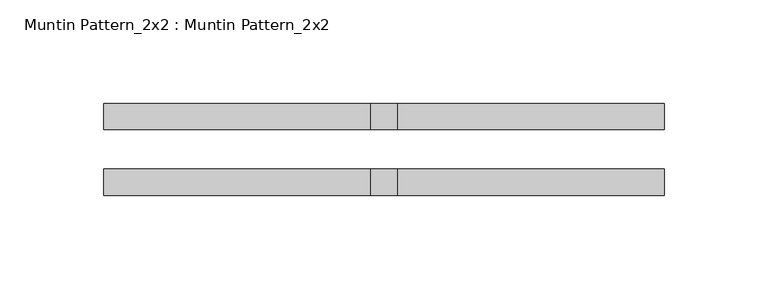
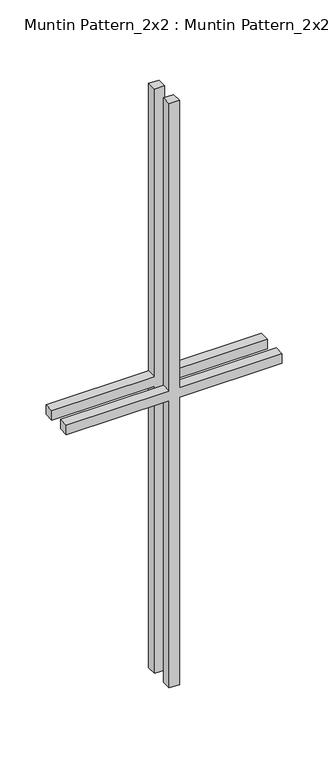
"""IFC4 building model written with IfcOpenShell, lengths in millimetres: proxy geometry, Muntin Pattern_2x2 : Muntin Pattern_2x2."""

from ifc_helpers import new_model, si_unit, frame, origin, place, context, project, spatial, polyline, outline, extrude, source, transform, mapped, element, save


def muntin_pattern_2x2_muntin_pattern_2x2_453f50af(model_context):
    return source(origin(), model_context, "Body", "SweptSolid", [
        extrude(outline(polyline([(393.7, -6.35), (393.7, -135.4666667), (381.0, -135.4666667), (381.0, -6.35), (0.0, -6.35), (0.0, 6.35), (381.0, 6.35), (381.0, 135.4666667), (393.7, 135.4666667), (393.7, 6.35), (774.7, 6.35), (774.7, -6.35), (393.7, -6.35)])), frame((0.0, 9.525, 0.0), z_axis=(0.0, 1.0, 0.0), x_axis=(0.0, 0.0, 1.0)), (0.0, 0.0, 1.0), 12.7),
        extrude(outline(polyline([(393.7, -6.35), (393.7, -135.4666667), (381.0, -135.4666667), (381.0, -6.35), (0.0, -6.35), (0.0, 6.35), (381.0, 6.35), (381.0, 135.4666667), (393.7, 135.4666667), (393.7, 6.35), (774.7, 6.35), (774.7, -6.35), (393.7, -6.35)])), frame((0.0, -22.225, 0.0), z_axis=(0.0, 1.0, 0.0), x_axis=(0.0, 0.0, 1.0)), (0.0, 0.0, 1.0), 12.7),
    ])


if __name__ == "__main__":
    model = new_model("IFC4")
    model_context = context("Model", 3, world=origin())
    ifc_project = project(units=[si_unit("LENGTHUNIT", "METRE", prefix="MILLI")], contexts=[model_context])
    site = spatial("IfcSite", under=ifc_project)
    building = spatial("IfcBuilding", under=site)
    placement = place(None, origin())
    muntin_pattern_2x2_muntin_pattern_2x2_shape = muntin_pattern_2x2_muntin_pattern_2x2_453f50af(model_context)
    element("IfcBuildingElementProxy", 1, Name="Muntin Pattern_2x2 : Muntin Pattern_2x2", ObjectType="Muntin Pattern_2x2 : Muntin Pattern_2x2", at=placement, inside=building, context=model_context, shape_type="MappedRepresentation", body=[
        mapped(muntin_pattern_2x2_muntin_pattern_2x2_shape, transform((0.0, 0.0, 0.0), x_axis=(1.0, 0.0, 0.0), y_axis=(0.0, 1.0, 0.0), z_axis=(0.0, 0.0, 1.0))),
    ])
    save(model, "model.ifc")

# Revit data of these elements
# Type "Muntin Pattern_2x2 : Muntin Pattern_2x2"
#   Width [instance default] = 4' - 0"
#   Thickness = 0' - 0 1/2"
#   Height [instance default] = 4' - 0"
#   Distance = 0' - 0 3/4"
#   Interior Material [instance default] = none
#   Exterior Material [instance default] = none
#   Default Elevation = 0
# Element 1 (IfcBuildingElementProxy, "Muntin Pattern_2x2 : Muntin Pattern_2x2")
#   Width = 0' - 10.66667"
#   Height = 2' - 6 1/2"
#   Interior Material = Wood - Stained
#   Exterior Material = Clad - White
#   Materials on its faces: "Clad - White", "Wood - Stained"
# Materials
#   "Clad - White": class "Wood", colour RGB 242 242 238, transparency 0, Cost = 0
#   "Wood - Stained": class "Wood", colour RGB 224 178 126, transparency 0, Cost = 0
